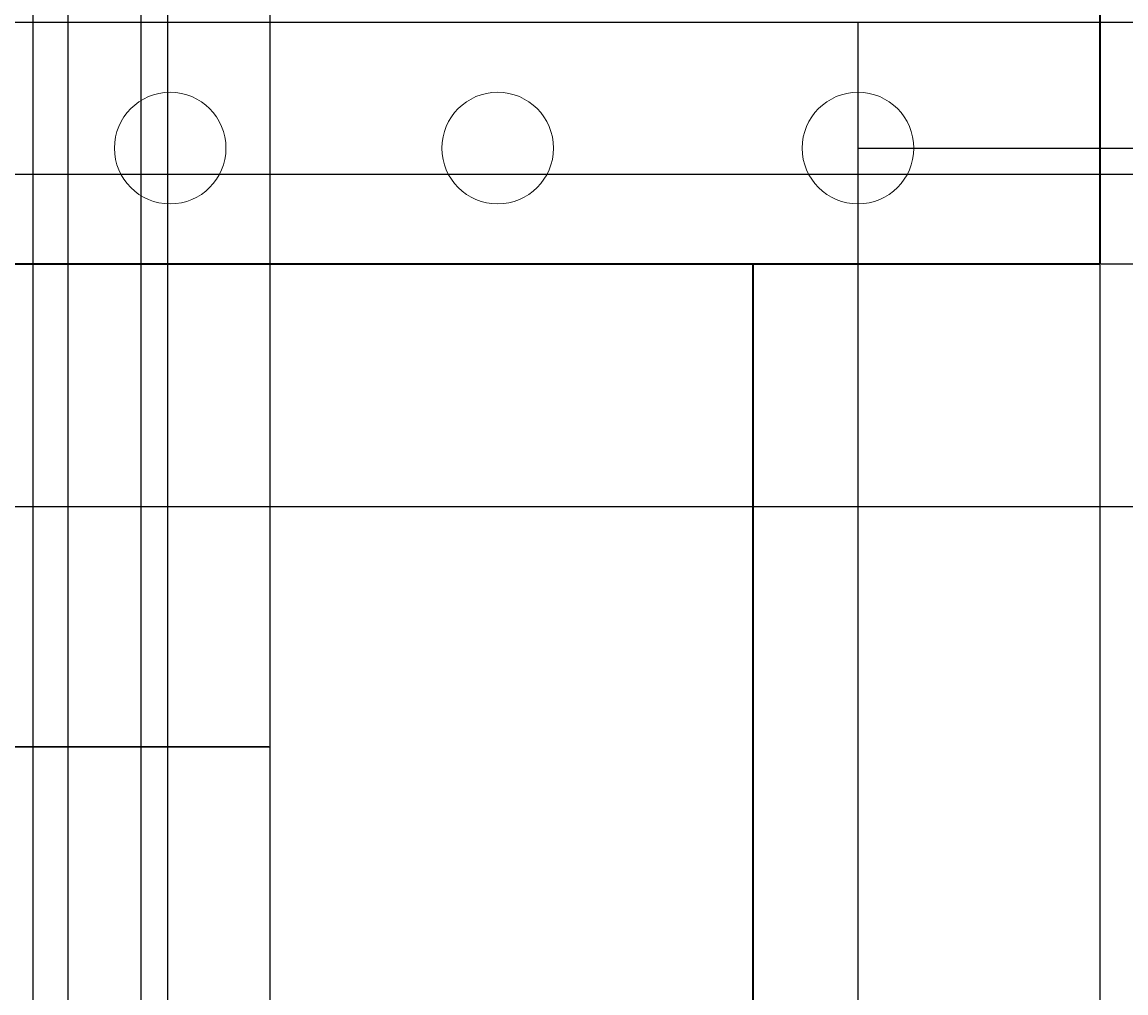
# Model space of a CAD drawing. Units: inches. Extents: x -13 to 809, y 112 to 656.
# Tile 13 of 55: x 257 to 339, y 252 to 325. Entities that reach past the tile are written whole.
import ezdxf

# ---------------------------------------------------------------- set-up
doc = ezdxf.new("R2010")
doc.units = ezdxf.units.IN
doc.header["$MEASUREMENT"] = 0
for name, color, linetype, lineweight in [('A-ANNO-DIMS', 2, 'Continuous', 18), ('A-ELEV', 7, 'Continuous', 35), ('A-ELEV-OTLN', 7, 'Continuous', 18), ('A-GLAZ', 4, 'Continuous', 25)]:
    doc.layers.add(name, color=color, linetype=linetype, lineweight=lineweight)
doc.styles.get("Standard").update_dxf_attribs({"font": 'arial.ttf'})
doc.dimstyles.get("Standard").update_dxf_attribs({"dimtxt": 0.625, "dimasz": 0.18, "dimexe": 0.18, "dimexo": 0.0625, "dimgap": 0.09, "dimtad": 0, "dimtih": 1, "dimtoh": 1, "dimdec": 4, "dimzin": 0, "dimdsep": 46, "dimlunit": 4, "dimtxsty": 'Standard', "dimcen": 0.09, "dimadec": 0, "dimazin": 0, "dimtfac": 1, "dimtdec": 4, "dimtofl": 0, "dimtmove": 0, "dimatfit": 3, "dimfxl": 1, "dimtolj": 1, "dimtzin": 0, "dimarcsym": 0})

# ---------------------------------------------------------------- blocks, each defined once
blk = doc.blocks.new('*D18')
at = {"layer": 'A-ANNO-DIMS', "color": 0, "lineweight": -2, "transparency": 16777216}
for p, q in [((337.507, 306.457), (337.507, 112.34)), ((311.463, 210.722), (311.463, 112.34)), ((311.643, 112.52), (323.09, 112.52)), ((337.327, 112.52), (325.88, 112.52))]:
    blk.add_line(p, q, dxfattribs=at)
at = {"layer": 'A-ANNO-DIMS', "color": 0, "transparency": 16777216}
for points in [[(311.643, 112.55), (311.643, 112.49), (311.463, 112.52)], [(337.327, 112.55), (337.327, 112.49), (337.507, 112.52)]]:
    blk.add_solid(points, dxfattribs=at)
at = {"layer": 'Defpoints', "color": 0, "transparency": 16777216}
for p in [(337.507, 306.52), (311.463, 210.785), (337.507, 112.52)]:
    blk.add_point(p, dxfattribs=at)
at = {"layer": 'A-ANNO-DIMS', "color": 0, "transparency": 16777216, "insert": (324.485, 112.52), "char_height": 0.625, "attachment_point": 5}
blk.add_mtext('\\A1;26.045', dxfattribs=at)
blk = doc.blocks.new('*D19')
at = {"layer": 'A-ANNO-DIMS', "color": 0, "lineweight": -2, "transparency": 16777216}
for p, q in [((337.507, 306.457), (337.507, 112.34)), ((365.938, 210.722), (365.938, 112.34)), ((337.687, 112.52), (350.573, 112.52)), ((365.758, 112.52), (352.873, 112.52))]:
    blk.add_line(p, q, dxfattribs=at)
at = {"layer": 'A-ANNO-DIMS', "color": 0, "transparency": 16777216}
for points in [[(337.687, 112.55), (337.687, 112.49), (337.507, 112.52)], [(365.758, 112.55), (365.758, 112.49), (365.938, 112.52)]]:
    blk.add_solid(points, dxfattribs=at)
at = {"layer": 'Defpoints', "color": 0, "transparency": 16777216}
for p in [(337.507, 306.52), (365.938, 210.785), (365.938, 112.52)]:
    blk.add_point(p, dxfattribs=at)
at = {"layer": 'A-ANNO-DIMS', "color": 0, "transparency": 16777216, "insert": (351.723, 112.52), "char_height": 0.625, "attachment_point": 5}
blk.add_mtext('\\A1;28.43', dxfattribs=at)
blk = doc.blocks.new('*D39')
at = {"layer": 'A-ANNO-DIMS', "color": 0, "lineweight": -2, "transparency": 16777216}
for p, q in [((341.345, 524.281), (-12.099, 524.281)), ((-11.919, 524.101), (-11.919, 406.775)), ((-11.919, 288.631), (-11.919, 405.957)), ((341.345, 288.451), (-12.099, 288.451))]:
    blk.add_line(p, q, dxfattribs=at)
at = {"layer": 'A-ANNO-DIMS', "color": 0, "transparency": 16777216}
for points in [[(-11.949, 524.101), (-11.889, 524.101), (-11.919, 524.281)], [(-11.949, 288.631), (-11.889, 288.631), (-11.919, 288.451)]]:
    blk.add_solid(points, dxfattribs=at)
at = {"layer": 'Defpoints', "color": 0, "transparency": 16777216}
for p in [(-11.919, 524.281), (341.407, 524.281), (341.407, 288.451)]:
    blk.add_point(p, dxfattribs=at)
at = {"layer": 'A-ANNO-DIMS', "color": 0, "transparency": 16777216, "insert": (-11.919, 406.366), "char_height": 0.625, "attachment_point": 5}
blk.add_mtext('\\A1;235.83', dxfattribs=at)
blk = doc.blocks.new('*D40')
at = {"layer": 'A-ANNO-DIMS', "color": 0, "lineweight": -2, "transparency": 16777216}
for p, q in [((471.037, 313.167), (-12.099, 313.167)), ((-11.919, 312.987), (-11.919, 301.218)), ((-11.919, 288.631), (-11.919, 300.4)), ((341.345, 288.451), (-12.099, 288.451))]:
    blk.add_line(p, q, dxfattribs=at)
at = {"layer": 'A-ANNO-DIMS', "color": 0, "transparency": 16777216}
for points in [[(-11.949, 312.987), (-11.889, 312.987), (-11.919, 313.167)], [(-11.949, 288.631), (-11.889, 288.631), (-11.919, 288.451)]]:
    blk.add_solid(points, dxfattribs=at)
at = {"layer": 'Defpoints', "color": 0, "transparency": 16777216}
for p in [(471.1, 313.167), (-11.919, 288.451), (341.407, 288.451)]:
    blk.add_point(p, dxfattribs=at)
at = {"layer": 'A-ANNO-DIMS', "color": 0, "transparency": 16777216, "insert": (-11.919, 300.809), "char_height": 0.625, "attachment_point": 5}
blk.add_mtext('\\A1;24.716', dxfattribs=at)
blk = doc.blocks.new('*D41')
at = {"layer": 'A-ANNO-DIMS', "color": 0, "lineweight": -2, "transparency": 16777216}
for p, q in [((471.037, 357.98), (-12.099, 357.98)), ((-11.919, 357.8), (-11.919, 335.983)), ((-11.919, 313.347), (-11.919, 335.164)), ((471.037, 313.167), (-12.099, 313.167))]:
    blk.add_line(p, q, dxfattribs=at)
at = {"layer": 'A-ANNO-DIMS', "color": 0, "transparency": 16777216}
for points in [[(-11.949, 357.8), (-11.889, 357.8), (-11.919, 357.98)], [(-11.949, 313.347), (-11.889, 313.347), (-11.919, 313.167)]]:
    blk.add_solid(points, dxfattribs=at)
at = {"layer": 'Defpoints', "color": 0, "transparency": 16777216}
for p in [(-11.919, 357.98), (471.1, 357.98), (471.1, 313.167)]:
    blk.add_point(p, dxfattribs=at)
at = {"layer": 'A-ANNO-DIMS', "color": 0, "transparency": 16777216, "insert": (-11.919, 335.574), "char_height": 0.625, "attachment_point": 5}
blk.add_mtext('\\A1;44.81', dxfattribs=at)
blk = doc.blocks.new('*D45')
at = {"layer": 'A-ANNO-DIMS', "color": 0, "lineweight": -2, "transparency": 16777216}
for p, q in [((275.652, 270.602), (-12.099, 270.602)), ((-11.919, 270.422), (-11.919, 247.259)), ((-11.919, 223.28), (-11.919, 246.443)), ((275.652, 223.1), (-12.099, 223.1))]:
    blk.add_line(p, q, dxfattribs=at)
at = {"layer": 'A-ANNO-DIMS', "color": 0, "transparency": 16777216}
for points in [[(-11.949, 270.422), (-11.889, 270.422), (-11.919, 270.602)], [(-11.949, 223.28), (-11.889, 223.28), (-11.919, 223.1)]]:
    blk.add_solid(points, dxfattribs=at)
at = {"layer": 'Defpoints', "color": 0, "transparency": 16777216}
for p in [(-11.919, 270.602), (275.715, 270.602), (275.715, 223.1)]:
    blk.add_point(p, dxfattribs=at)
at = {"layer": 'A-ANNO-DIMS', "color": 0, "transparency": 16777216, "insert": (-11.919, 246.851), "char_height": 0.625, "attachment_point": 5}
blk.add_mtext('\\A1;47.5', dxfattribs=at)
blk = doc.blocks.new('*D46')
at = {"layer": 'A-ANNO-DIMS', "color": 0, "lineweight": -2, "transparency": 16777216}
for p, q in [((160.981, 408.794), (807.769, 408.794)), ((807.589, 408.614), (807.589, 367.066)), ((807.589, 324.7), (807.589, 366.248)), ((160.981, 324.52), (807.769, 324.52))]:
    blk.add_line(p, q, dxfattribs=at)
at = {"layer": 'A-ANNO-DIMS', "color": 0, "transparency": 16777216}
for points in [[(807.559, 408.614), (807.619, 408.614), (807.589, 408.794)], [(807.559, 324.7), (807.619, 324.7), (807.589, 324.52)]]:
    blk.add_solid(points, dxfattribs=at)
at = {"layer": 'Defpoints', "color": 0, "transparency": 16777216}
for p in [(160.918, 408.794), (807.589, 408.794), (160.918, 324.52)]:
    blk.add_point(p, dxfattribs=at)
at = {"layer": 'A-ANNO-DIMS', "color": 0, "transparency": 16777216, "insert": (807.589, 366.657), "char_height": 0.625, "attachment_point": 5}
blk.add_mtext('\\A1;84.27', dxfattribs=at)
blk = doc.blocks.new('*D48')
at = {"layer": 'A-ANNO-DIMS', "color": 0, "lineweight": -2, "transparency": 16777216}
for p, q in [((319.57, 444.52), (807.769, 444.52)), ((807.589, 444.34), (807.589, 384.929)), ((807.589, 324.7), (807.589, 384.111)), ((319.57, 324.52), (807.769, 324.52))]:
    blk.add_line(p, q, dxfattribs=at)
at = {"layer": 'A-ANNO-DIMS', "color": 0, "transparency": 16777216}
for points in [[(807.559, 444.34), (807.619, 444.34), (807.589, 444.52)], [(807.559, 324.7), (807.619, 324.7), (807.589, 324.52)]]:
    blk.add_solid(points, dxfattribs=at)
at = {"layer": 'Defpoints', "color": 0, "transparency": 16777216}
for p in [(319.507, 444.52), (807.589, 444.52), (319.507, 324.52)]:
    blk.add_point(p, dxfattribs=at)
at = {"layer": 'A-ANNO-DIMS', "color": 0, "transparency": 16777216, "insert": (807.589, 384.52), "char_height": 0.625, "attachment_point": 5}
blk.add_mtext('\\A1;120', dxfattribs=at)
blk = doc.blocks.new('*D106')
at = {"layer": 'A-ANNO-DIMS', "color": 0, "lineweight": -2, "transparency": 16777216}
for p, q in [((319.57, 315.144), (807.769, 315.144)), ((807.589, 314.964), (807.589, 311.241)), ((807.589, 306.7), (807.589, 310.423)), ((337.57, 306.52), (807.769, 306.52))]:
    blk.add_line(p, q, dxfattribs=at)
at = {"layer": 'A-ANNO-DIMS', "color": 0, "transparency": 16777216}
for points in [[(807.559, 314.964), (807.619, 314.964), (807.589, 315.144)], [(807.559, 306.7), (807.619, 306.7), (807.589, 306.52)]]:
    blk.add_solid(points, dxfattribs=at)
at = {"layer": 'Defpoints', "color": 0, "transparency": 16777216}
for p in [(319.507, 315.144), (807.589, 315.144), (337.507, 306.52)]:
    blk.add_point(p, dxfattribs=at)
at = {"layer": 'A-ANNO-DIMS', "color": 0, "transparency": 16777216, "insert": (807.589, 310.832), "char_height": 0.625, "attachment_point": 5}
blk.add_mtext('\\A1;8.624', dxfattribs=at)
blk = doc.blocks.new('*D108')
at = {"layer": 'A-ANNO-DIMS', "color": 0, "lineweight": -2, "transparency": 16777216}
for p, q in [((319.507, 324.457), (319.507, 112.34)), ((337.507, 306.457), (337.507, 112.34)), ((319.687, 112.52), (327.393, 112.52)), ((337.327, 112.52), (329.621, 112.52))]:
    blk.add_line(p, q, dxfattribs=at)
at = {"layer": 'A-ANNO-DIMS', "color": 0, "transparency": 16777216}
for points in [[(319.687, 112.55), (319.687, 112.49), (319.507, 112.52)], [(337.327, 112.55), (337.327, 112.49), (337.507, 112.52)]]:
    blk.add_solid(points, dxfattribs=at)
at = {"layer": 'Defpoints', "color": 0, "transparency": 16777216}
for p in [(319.507, 324.52), (337.507, 306.52), (337.507, 112.52)]:
    blk.add_point(p, dxfattribs=at)
at = {"layer": 'A-ANNO-DIMS', "color": 0, "transparency": 16777216, "insert": (328.507, 112.52), "char_height": 0.625, "attachment_point": 5}
blk.add_mtext('\\A1;18.00', dxfattribs=at)
blk = doc.blocks.new('*D112')
at = {"layer": 'A-ANNO-DIMS', "color": 0, "lineweight": -2, "transparency": 16777216}
for p, q in [((210.079, 361.229), (210.079, 112.34)), ((275.715, 361.229), (275.715, 112.34)), ((210.259, 112.52), (241.752, 112.52)), ((275.535, 112.52), (244.042, 112.52))]:
    blk.add_line(p, q, dxfattribs=at)
at = {"layer": 'A-ANNO-DIMS', "color": 0, "transparency": 16777216}
for points in [[(210.259, 112.55), (210.259, 112.49), (210.079, 112.52)], [(275.535, 112.55), (275.535, 112.49), (275.715, 112.52)]]:
    blk.add_solid(points, dxfattribs=at)
at = {"layer": 'Defpoints', "color": 0, "transparency": 16777216}
for p in [(210.079, 361.292), (275.715, 361.292), (275.715, 112.52)]:
    blk.add_point(p, dxfattribs=at)
at = {"layer": 'A-ANNO-DIMS', "color": 0, "transparency": 16777216, "insert": (242.897, 112.52), "char_height": 0.625, "attachment_point": 5}
blk.add_mtext('\\A1;65.64', dxfattribs=at)
blk = doc.blocks.new('*D113')
at = {"layer": 'A-ANNO-DIMS', "color": 0, "lineweight": -2, "transparency": 16777216}
for p, q in [((275.715, 361.229), (275.715, 112.34)), ((319.507, 324.457), (319.507, 112.34)), ((275.895, 112.52), (296.453, 112.52)), ((319.327, 112.52), (298.769, 112.52))]:
    blk.add_line(p, q, dxfattribs=at)
at = {"layer": 'A-ANNO-DIMS', "color": 0, "transparency": 16777216}
for points in [[(275.895, 112.55), (275.895, 112.49), (275.715, 112.52)], [(319.327, 112.55), (319.327, 112.49), (319.507, 112.52)]]:
    blk.add_solid(points, dxfattribs=at)
at = {"layer": 'Defpoints', "color": 0, "transparency": 16777216}
for p in [(275.715, 361.292), (319.507, 324.52), (319.507, 112.52)]:
    blk.add_point(p, dxfattribs=at)
at = {"layer": 'A-ANNO-DIMS', "color": 0, "transparency": 16777216, "insert": (297.611, 112.52), "char_height": 0.625, "attachment_point": 5}
blk.add_mtext('\\A1;43.79', dxfattribs=at)
blk = doc.blocks.new('*D116')
at = {"layer": 'A-ANNO-DIMS', "color": 0, "lineweight": -2, "transparency": 16777216}
for p, q in [((258.102, 210.847), (258.102, 655.963)), ((260.705, 207.435), (260.705, 655.963)), ((258.282, 655.783), (258.497, 655.783)), ((260.525, 655.783), (260.309, 655.783))]:
    blk.add_line(p, q, dxfattribs=at)
at = {"layer": 'A-ANNO-DIMS', "color": 0, "transparency": 16777216}
for points in [[(258.282, 655.813), (258.282, 655.753), (258.102, 655.783)], [(260.525, 655.813), (260.525, 655.753), (260.705, 655.783)]]:
    blk.add_solid(points, dxfattribs=at)
at = {"layer": 'Defpoints', "color": 0, "transparency": 16777216}
for p in [(260.705, 655.783), (258.102, 210.785), (260.705, 207.372)]:
    blk.add_point(p, dxfattribs=at)
at = {"layer": 'A-ANNO-DIMS', "color": 0, "transparency": 16777216, "insert": (259.403, 655.783), "char_height": 0.625, "attachment_point": 5}
blk.add_mtext('\\A1;2.60', dxfattribs=at)
blk = doc.blocks.new('*D119')
at = {"layer": 'A-ANNO-DIMS', "color": 0, "lineweight": -2, "transparency": 16777216}
for p, q in [((266.1286, 207.43492), (266.1286, 655.962835)), ((268.1286, 207.43492), (268.1286, 655.962835)), ((265.9486, 655.782835), (265.7686, 655.782835)), ((268.3086, 655.782835), (268.4886, 655.782835))]:
    blk.add_line(p, q, dxfattribs=at)
at = {"layer": 'A-ANNO-DIMS', "color": 0, "transparency": 16777216}
for points in [[(265.9486, 655.812835), (265.9486, 655.752835), (266.1286, 655.782835)], [(268.3086, 655.812835), (268.3086, 655.752835), (268.1286, 655.782835)]]:
    blk.add_solid(points, dxfattribs=at)
at = {"layer": 'Defpoints', "color": 0, "transparency": 16777216}
for p in [(268.1286, 655.782835), (266.1286, 207.37242), (268.1286, 207.37242)]:
    blk.add_point(p, dxfattribs=at)
at = {"layer": 'A-ANNO-DIMS', "color": 0, "transparency": 16777216, "insert": (267.1286, 655.782835), "char_height": 0.625, "attachment_point": 5}
blk.add_mtext('\\A1;2.00', dxfattribs=at)

msp = doc.modelspace()

# ---------------------------------------------------------------- linework, layer by layer
at = {"layer": 'A-ELEV'}
for p, q in [((337.5074, 462.5199), (337.5074, 306.5199)), ((109.5888, 306.5199), (337.5074, 306.5199)), ((311.6991, 210.4452), (311.6991, 306.5199))]:
    msp.add_line(p, q, dxfattribs=at)
at = {"layer": 'A-ELEV-OTLN'}
for centre in [(268.3019, 315.1435), (292.6832, 315.1435), (319.5074, 315.1435)]:
    msp.add_circle(centre, 4.1542, dxfattribs=at)
at = {"layer": 'A-GLAZ'}
msp.add_lwpolyline([(210.0791, 270.6024), (275.7145, 270.6024), (275.7145, 223.1), (210.0791, 223.1)], close=True, dxfattribs=at)

# ---------------------------------------------------------------- dimensions: what is measured, and where the dimension line sits
at = {"layer": 'A-ANNO-DIMS'}
for base, p1, p2, override, picture, middle in [((260.7048, 655.7828), (258.1022, 210.7849), (260.7048, 207.3724), {"dimdec": 2, "dimlfac": 1, "dimrnd": 0, "dimzin": 0, "dimdsep": 46, "dimlunit": 2}, '*D116', (259.4035, 655.7828)), ((268.1286, 655.7828), (266.1286, 207.3724), (268.1286, 207.3724), {"dimdec": 2, "dimlfac": 1, "dimrnd": 0, "dimzin": 0, "dimdsep": 46, "dimlunit": 2}, '*D119', (267.1286, 655.7828)), ((275.7145, 112.5199), (210.0791, 361.2915), (275.7145, 361.2915), {"dimdec": 2, "dimlfac": 1, "dimrnd": 0, "dimzin": 0, "dimdsep": 46, "dimlunit": 2}, '*D112', (242.8968, 112.5199)), ((319.5074, 112.5199), (275.7145, 361.2915), (319.5074, 324.5199), {"dimdec": 2, "dimlfac": 1, "dimrnd": 0, "dimzin": 0, "dimdsep": 46, "dimlunit": 2}, '*D113', (297.611, 112.5199)), ((337.5074, 112.5199), (319.5074, 324.5199), (337.5074, 306.5199), {"dimdec": 2, "dimlfac": 1, "dimrnd": 0, "dimzin": 0, "dimdsep": 46, "dimlunit": 2}, '*D108', (328.5074, 112.5199)), ((337.5074, 112.5199), (311.4627, 210.7849), (337.5074, 306.5199), {"dimdec": 3, "dimlfac": 1, "dimrnd": 0, "dimzin": 0, "dimdsep": 46, "dimlunit": 2}, '*D18', (324.4851, 112.5199)), ((365.9383, 112.5199), (337.5074, 306.5199), (365.9383, 210.7849), {"dimdec": 2, "dimlfac": 1, "dimrnd": 0, "dimzin": 0, "dimdsep": 46, "dimlunit": 2}, '*D19', (351.7228, 112.5199))]:
    dim = msp.add_linear_dim(base=base, p1=p1, p2=p2, dimstyle='Standard', override=override, dxfattribs=at)
    dim.commit()
    dim.dimension.update_dxf_attribs({"geometry": picture, "text_midpoint": middle})
for base, p1, p2, override, picture, middle in [((-11.9191, 524.281), (341.4072, 288.4508), (341.4072, 524.281), {"dimdec": 2, "dimlfac": 1, "dimrnd": 0, "dimzin": 0, "dimdsep": 46, "dimlunit": 2}, '*D39', (-11.9191, 406.3659)), ((807.5888, 444.5199), (319.5074, 324.5199), (319.5074, 444.5199), {"dimdec": 0, "dimlfac": 1, "dimrnd": 0, "dimzin": 0, "dimdsep": 46, "dimlunit": 2}, '*D48', (807.5888, 384.5199)), ((807.5888, 408.7939), (160.9184, 324.5199), (160.9184, 408.7939), {"dimdec": 2, "dimlfac": 1, "dimrnd": 0, "dimzin": 0, "dimdsep": 46, "dimlunit": 2}, '*D46', (807.5888, 366.6569)), ((-11.9191, 357.9804), (471.0998, 313.1667), (471.0998, 357.9804), {"dimdec": 2, "dimlfac": 1, "dimrnd": 0, "dimzin": 0, "dimdsep": 46, "dimlunit": 2}, '*D41', (-11.9191, 335.5735)), ((807.5888, 315.1435), (337.5074, 306.5199), (319.5074, 315.1435), {"dimdec": 3, "dimlfac": 1, "dimrnd": 0, "dimzin": 0, "dimdsep": 46, "dimlunit": 2}, '*D106', (807.5888, 310.8317)), ((-11.9191, 288.4508), (471.0998, 313.1667), (341.4072, 288.4508), {"dimdec": 3, "dimlfac": 1, "dimrnd": 0, "dimzin": 0, "dimdsep": 46, "dimlunit": 2}, '*D40', (-11.9191, 300.8087)), ((-11.9191, 270.6024), (275.7145, 223.1), (275.7145, 270.6024), {"dimdec": 1, "dimlfac": 1, "dimrnd": 0, "dimzin": 0, "dimdsep": 46, "dimlunit": 2}, '*D45', (-11.9191, 246.8512))]:
    dim = msp.add_linear_dim(base=base, p1=p1, p2=p2, angle=90, dimstyle='Standard', override=override, dxfattribs=at)
    dim.commit()
    dim.dimension.update_dxf_attribs({"geometry": picture, "text_midpoint": middle})

doc.saveas('drawing.dxf')
